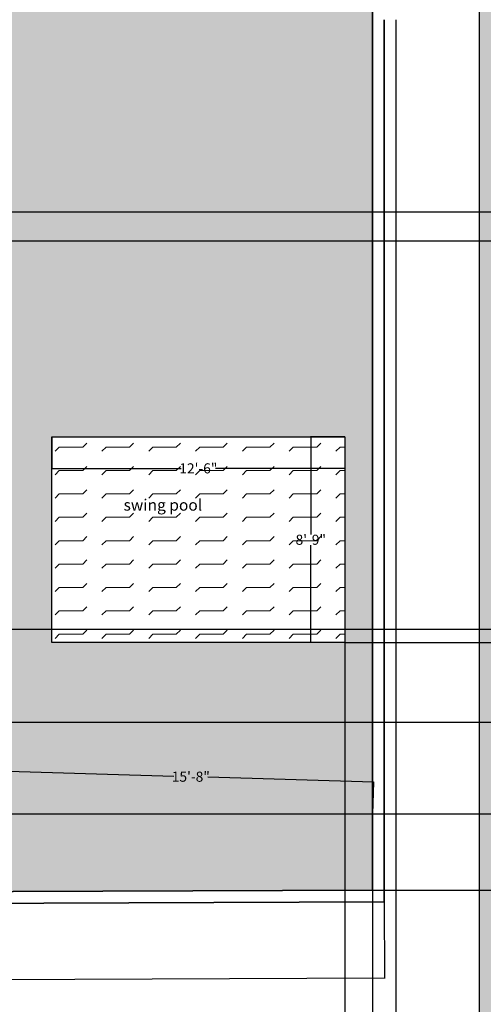
# Model space of a CAD drawing. Units: inches. Extents: x -157 to 1464, y -361 to 1077.
# Tile 7 of 9: x 676 to 913, y 14 to 519. Entities that reach past the tile are written whole.
import ezdxf

# ---------------------------------------------------------------- set-up
doc = ezdxf.new("R2010")
doc.units = ezdxf.units.IN
doc.header["$MEASUREMENT"] = 0
for name, color, linetype, lineweight in [('A-ANNO-DIMS', 2, 'Continuous', 18), ('C-ANNO-DIMS', 2, 'Continuous', 18), ('C-ANNO-TEXT', 7, 'Continuous', 18), ('C-POOL-PATT', 143, 'Continuous', 13), ('C-PROP', 7, 'Continuous', 35), ('C-ROAD', 7, 'Continuous', 25), ('C-ROAD-PATT', 8, 'Continuous', 13), ('C-SITE-POOL', 4, 'Continuous', 25), ('L-GRND-PATT', 8, 'Continuous', 13)]:
    doc.layers.add(name, color=color, linetype=linetype, lineweight=lineweight)
doc.styles.get("Standard").update_dxf_attribs({"font": 'arial.ttf'})
doc.dimstyles.new('Annotative', dxfattribs={"dimscale": 0, "dimtxt": 5.18, "dimasz": 0.18, "dimexe": 0.18, "dimexo": 0.0625, "dimgap": 0.09, "dimtad": 0, "dimtih": 1, "dimtoh": 1, "dimdec": 0, "dimzin": 0, "dimdsep": 46, "dimlunit": 3, "dimtxsty": 'Standard', "dimcen": 0.09, "dimadec": 0, "dimazin": 0, "dimtfac": 1, "dimtdec": 0, "dimtofl": 0, "dimtmove": 0, "dimatfit": 3, "dimfxl": 1, "dimtolj": 1, "dimtzin": 0, "dimarcsym": 0})

# ---------------------------------------------------------------- blocks, each defined once
blk = doc.blocks.new('*D14')
at = {"layer": 'C-ANNO-DIMS', "color": 0, "lineweight": -2, "transparency": 16777216}
for p, q in [((862.57, 66.62), (862.72, 27.26)), ((251.33, 64.28), (251.48, 24.92)), ((251.66, 25.1), (546.1, 26.23)), ((862.54, 27.44), (568.1, 26.31))]:
    blk.add_line(p, q, dxfattribs=at)
at = {"layer": 'C-ANNO-DIMS', "color": 0, "transparency": 16777216}
for points in [[(862.54, 27.47), (862.54, 27.41), (862.72, 27.44)], [(251.66, 25.13), (251.66, 25.07), (251.48, 25.1)]]:
    blk.add_solid(points, dxfattribs=at)
at = {"layer": 'Defpoints', "color": 0, "transparency": 16777216}
for p in [(862.57, 66.68), (251.33, 64.34), (862.72, 27.44)]:
    blk.add_point(p, dxfattribs=at)
at = {"layer": 'C-ANNO-DIMS', "color": 0, "transparency": 16777216, "insert": (557.1, 26.27), "char_height": 5.18, "attachment_point": 5}
blk.add_mtext('\\A1;50\'-11"', dxfattribs=at)
blk = doc.blocks.new('*D15')
at = {"layer": 'C-ANNO-DIMS', "color": 0, "lineweight": -2, "transparency": 16777216}
for p, q in [((692.18, 305.18), (692.18, 288.97)), ((842.44, 305.18), (842.44, 288.97)), ((692.36, 289.15), (758.57, 289.15)), ((842.26, 289.15), (776.05, 289.15))]:
    blk.add_line(p, q, dxfattribs=at)
at = {"layer": 'C-ANNO-DIMS', "color": 0, "transparency": 16777216}
for points in [[(692.36, 289.18), (692.36, 289.12), (692.18, 289.15)], [(842.26, 289.18), (842.26, 289.12), (842.44, 289.15)]]:
    blk.add_solid(points, dxfattribs=at)
at = {"layer": 'Defpoints', "color": 0, "transparency": 16777216}
for p in [(692.18, 305.24), (842.44, 305.24), (842.44, 289.15)]:
    blk.add_point(p, dxfattribs=at)
at = {"layer": 'C-ANNO-DIMS', "color": 0, "transparency": 16777216, "insert": (767.31, 289.15), "char_height": 5.18, "attachment_point": 5}
blk.add_mtext('\\A1;12\'-6"', dxfattribs=at)
blk = doc.blocks.new('*D16')
at = {"layer": 'C-ANNO-DIMS', "color": 0, "lineweight": -2, "transparency": 16777216}
for p, q in [((842.38, 305.24), (824.79, 305.24)), ((824.97, 305.06), (824.97, 255.24)), ((824.97, 199.96), (824.97, 249.77)), ((842.38, 199.78), (824.79, 199.78))]:
    blk.add_line(p, q, dxfattribs=at)
at = {"layer": 'C-ANNO-DIMS', "color": 0, "transparency": 16777216}
for points in [[(824.94, 305.06), (825, 305.06), (824.97, 305.24)], [(824.94, 199.96), (825, 199.96), (824.97, 199.78)]]:
    blk.add_solid(points, dxfattribs=at)
at = {"layer": 'Defpoints', "color": 0, "transparency": 16777216}
for p in [(842.44, 305.24), (824.97, 199.78), (842.44, 199.78)]:
    blk.add_point(p, dxfattribs=at)
at = {"layer": 'C-ANNO-DIMS', "color": 0, "transparency": 16777216, "insert": (824.97, 252.51), "char_height": 5.18, "attachment_point": 5}
blk.add_mtext('\\A1;8\'-9"', dxfattribs=at)
blk = doc.blocks.new('*D56')
at = {"layer": 'C-ANNO-DIMS', "color": 0, "lineweight": -2, "transparency": 16777216}
for p, q in [((668.97, 111.92), (669.64, 133.96)), ((669.82, 133.77), (754.7, 131.17)), ((857.06, 128.03), (772.18, 130.63)), ((856.57, 106.17), (857.25, 128.21))]:
    blk.add_line(p, q, dxfattribs=at)
at = {"layer": 'C-ANNO-DIMS', "color": 0, "transparency": 16777216}
for points in [[(669.82, 133.8), (669.82, 133.74), (669.64, 133.78)], [(857.06, 128.06), (857.06, 128), (857.24, 128.03)]]:
    blk.add_solid(points, dxfattribs=at)
at = {"layer": 'Defpoints', "color": 0, "transparency": 16777216}
for p in [(857.24, 128.03), (668.97, 111.86), (856.57, 106.11)]:
    blk.add_point(p, dxfattribs=at)
at = {"layer": 'C-ANNO-DIMS', "color": 0, "transparency": 16777216, "insert": (763.44, 130.9), "char_height": 5.18, "attachment_point": 5}
blk.add_mtext('\\A1;15\'-8"', dxfattribs=at)
blk = doc.blocks.new('*D64')
at = {"layer": 'A-ANNO-DIMS', "color": 0, "lineweight": -2, "transparency": 16777216}
for p, q in [((842.44, 199.71), (842.44, -357.73)), ((856.57, 72.59), (856.57, -357.73)), ((842.62, -357.55), (842.77, -357.55)), ((856.39, -357.55), (856.24, -357.55))]:
    blk.add_line(p, q, dxfattribs=at)
at = {"layer": 'A-ANNO-DIMS', "color": 0, "transparency": 16777216}
for points in [[(842.62, -357.52), (842.62, -357.58), (842.44, -357.55)], [(856.39, -357.52), (856.39, -357.58), (856.57, -357.55)]]:
    blk.add_solid(points, dxfattribs=at)
at = {"layer": 'Defpoints', "color": 0, "transparency": 16777216}
for p in [(842.44, 199.78), (856.57, 72.66), (856.57, -357.55)]:
    blk.add_point(p, dxfattribs=at)
at = {"layer": 'A-ANNO-DIMS', "color": 0, "transparency": 16777216, "insert": (849.51, -357.55), "char_height": 5.18, "attachment_point": 5}
blk.add_mtext('\\A1;1\'-2"', dxfattribs=at)
blk = doc.blocks.new('*D65')
at = {"layer": 'A-ANNO-DIMS', "color": 0, "lineweight": -2, "transparency": 16777216}
for p, q in [((842.5, 199.78), (1397.57, 199.78)), ((1397.39, 199.6), (1397.39, 138.95)), ((1397.39, 72.84), (1397.39, 133.48)), ((856.63, 72.66), (1397.57, 72.66))]:
    blk.add_line(p, q, dxfattribs=at)
at = {"layer": 'A-ANNO-DIMS', "color": 0, "transparency": 16777216}
for points in [[(1397.36, 199.6), (1397.42, 199.6), (1397.39, 199.78)], [(1397.36, 72.84), (1397.42, 72.84), (1397.39, 72.66)]]:
    blk.add_solid(points, dxfattribs=at)
at = {"layer": 'Defpoints', "color": 0, "transparency": 16777216}
for p in [(842.44, 199.78), (856.57, 72.66), (1397.39, 72.66)]:
    blk.add_point(p, dxfattribs=at)
at = {"layer": 'A-ANNO-DIMS', "color": 0, "transparency": 16777216, "insert": (1397.39, 136.22), "char_height": 5.18, "attachment_point": 5}
blk.add_mtext('\\A1;10\'-7"', dxfattribs=at)
blk = doc.blocks.new('*D69')
at = {"layer": 'A-ANNO-DIMS', "color": 0, "lineweight": -2, "transparency": 16777216}
for p, q in [((856.57, 519.36), (856.57, -357.73)), ((868.57, 519.36), (868.57, -357.73)), ((856.75, -357.55), (868.39, -357.55)), ((868.57, -357.55), (868.75, -357.55))]:
    blk.add_line(p, q, dxfattribs=at)
at = {"layer": 'A-ANNO-DIMS', "color": 0, "transparency": 16777216}
for points in [[(856.75, -357.52), (856.75, -357.58), (856.57, -357.55)], [(868.39, -357.52), (868.39, -357.58), (868.57, -357.55)]]:
    blk.add_solid(points, dxfattribs=at)
at = {"layer": 'Defpoints', "color": 0, "transparency": 16777216}
for p in [(856.57, 519.42), (868.57, 519.42), (868.57, -357.55)]:
    blk.add_point(p, dxfattribs=at)
at = {"layer": 'A-ANNO-DIMS', "color": 0, "transparency": 16777216, "insert": (875.48, -357.55), "char_height": 5.18, "attachment_point": 5}
blk.add_mtext('\\A1;1\'-0"', dxfattribs=at)
blk = doc.blocks.new('*D74')
at = {"layer": 'A-ANNO-DIMS', "color": 0, "lineweight": -2, "transparency": 16777216}
for p, q in [((597.03, 158.9), (1397.57, 158.9)), ((1397.39, 158.72), (1397.39, 138.11)), ((1397.39, 112.04), (1397.39, 132.64)), ((597.03, 111.86), (1397.57, 111.86))]:
    blk.add_line(p, q, dxfattribs=at)
at = {"layer": 'A-ANNO-DIMS', "color": 0, "transparency": 16777216}
for points in [[(1397.36, 158.72), (1397.42, 158.72), (1397.39, 158.9)], [(1397.36, 112.04), (1397.42, 112.04), (1397.39, 111.86)]]:
    blk.add_solid(points, dxfattribs=at)
at = {"layer": 'Defpoints', "color": 0, "transparency": 16777216}
for p in [(596.97, 158.9), (1397.39, 158.9), (596.97, 111.86)]:
    blk.add_point(p, dxfattribs=at)
at = {"layer": 'A-ANNO-DIMS', "color": 0, "transparency": 16777216, "insert": (1397.39, 135.38), "char_height": 5.18, "attachment_point": 5}
blk.add_mtext('\\A1;3\'-11"', dxfattribs=at)
blk = doc.blocks.new('*D76')
at = {"layer": 'A-ANNO-DIMS', "color": 0, "lineweight": -2, "transparency": 16777216}
for p, q in [((597.03, 420.86), (1397.57, 420.86)), ((1397.39, 420.68), (1397.39, 416.1)), ((1397.39, 406.04), (1397.39, 410.62)), ((597.03, 405.86), (1397.57, 405.86))]:
    blk.add_line(p, q, dxfattribs=at)
at = {"layer": 'A-ANNO-DIMS', "color": 0, "transparency": 16777216}
for points in [[(1397.36, 420.68), (1397.42, 420.68), (1397.39, 420.86)], [(1397.36, 406.04), (1397.42, 406.04), (1397.39, 405.86)]]:
    blk.add_solid(points, dxfattribs=at)
at = {"layer": 'Defpoints', "color": 0, "transparency": 16777216}
for p in [(596.97, 420.86), (1397.39, 420.86), (596.97, 405.86)]:
    blk.add_point(p, dxfattribs=at)
at = {"layer": 'A-ANNO-DIMS', "color": 0, "transparency": 16777216, "insert": (1397.39, 413.36), "char_height": 5.18, "attachment_point": 5}
blk.add_mtext('\\A1;1\'-3"', dxfattribs=at)
blk = doc.blocks.new('*D83')
at = {"layer": 'A-ANNO-DIMS', "color": 0, "lineweight": -2, "transparency": 16777216}
for p, q in [((652.31, 206.63), (1397.57, 206.63)), ((1397.39, 206.45), (1397.39, 161.94)), ((1397.39, 112.04), (1397.39, 156.56)), ((597.03, 111.86), (1397.57, 111.86))]:
    blk.add_line(p, q, dxfattribs=at)
at = {"layer": 'A-ANNO-DIMS', "color": 0, "transparency": 16777216}
for points in [[(1397.36, 206.45), (1397.42, 206.45), (1397.39, 206.63)], [(1397.36, 112.04), (1397.42, 112.04), (1397.39, 111.86)]]:
    blk.add_solid(points, dxfattribs=at)
at = {"layer": 'Defpoints', "color": 0, "transparency": 16777216}
for p in [(652.25, 206.63), (1397.39, 206.63), (596.97, 111.86)]:
    blk.add_point(p, dxfattribs=at)
at = {"layer": 'A-ANNO-DIMS', "color": 0, "transparency": 16777216, "insert": (1397.39, 159.25), "char_height": 5.18, "attachment_point": 5}
blk.add_mtext('\\A1;7\'-11"', dxfattribs=at)

msp = doc.modelspace()

# ---------------------------------------------------------------- hatches: boundary and pattern name
at = {"layer": 'C-POOL-PATT'}
h = msp.add_hatch(dxfattribs=at)
h.set_pattern_fill('FLEX', color=256, scale=48)
h.paths.add_polyline_path([(842.44, 305.24), (692.18, 305.24), (692.18, 199.78), (842.44, 199.78)])
at = {"layer": 'C-ROAD-PATT'}
h = msp.add_hatch(color=256, dxfattribs=at)
h.dxf.hatch_style = 1
h.paths.add_polyline_path([(1091.28, 858.84), (31.23, 858.84), (31.23, 838.38), (161.57, 774.56), (996.76, 774.56), (996.76, -105.32), (1027.51, -42.52), (1027.51, -185.11), (1027.51, -287.61), (1091.28, -186.19)])
h.paths.add_polyline_path([(899.55, 208.71), (1098.57, 208.71), (1098.57, 279.4), (899.55, 279.4)], flags=9)
h = msp.add_hatch(color=256, dxfattribs=at)
h.dxf.hatch_style = 1
h.paths.add_polyline_path([(990.76, 768.56), (31.23, 768.56), (-71.27, 768.56), (31.23, 704.11), (31.23, 678.84), (911.28, 678.84), (911.28, -185.11), (957.69, -185.11), (990.76, -117.57)])
h.paths.add_polyline_path([(899.55, 208.71), (1098.57, 208.71), (1098.57, 279.4), (899.55, 279.4)], flags=9)
h.paths.add_polyline_path([(645.57, 707.88), (844.59, 707.88), (844.59, 778.57), (645.57, 778.57)], flags=9)
h.paths.add_polyline_path([(892.1, 580.27), (940.38, 580.27), (940.38, 592.3), (892.1, 592.3)], flags=25)
at = {"layer": 'L-GRND-PATT'}
h = msp.add_hatch(dxfattribs=at)
h.set_pattern_fill('GRAVEL', color=256, scale=26)
h.set_pattern_definition([(228.01279, (18.72, 26), (-208, -234), [3.49794, -346.2963]), (184.96974, (16.38, 23.4), (312, 26), [6.00257, -594.25404]), (132.51045, (10.4, 22.88), (260, -286), [4.2325, -419.01685]), (267.27369, (0.26, 16.38), (26, 520), [5.4662, -541.1525]), (292.83365, (0, 10.92), (-130, 312), [5.36003, -530.6437]), (357.27369, (2.08, 5.98), (-520, 26), [5.4662, -541.1525]), (37.69424, (7.54, 5.72), (-338, -260), [7.22875, -715.64606]), (72.25533, (13.26, 10.14), (182, 572), [6.8247, -675.64436]), (121.42957, (15.34, 16.64), (-208, 338), [5.4847, -542.9859]), (175.23636, (12.48, 21.32), (286, -26), [6.26163, -306.81983]), (222.39744, (6.24, 21.84), (-312, -286), [8.09765, -801.66775]), (138.81407, (26, 16.12), (-182, 156), [2.76383, -273.61997]), (171.46923, (23.92, 17.94), (338, -52), [5.25816, -520.5593]), (225, (18.72, 18.72), (-3e-15, -26), [3.67695, -33.0926]), (203.1986, (16.9, 21.84), (130, 52), [1.9801, -196.03]), (291.8014, (15.08, 21.06), (-26, 78), [2.8003, -137.214]), (30.96376, (16.12, 18.46), (78, 52), [4.54815, -147.0566]), (161.56505, (20.02, 20.8), (52, -26), [3.28877, -78.93045]), (16.38954, (0, 21.06), (260, 78), [4.6072, -456.11397]), (70.34618, (4.42, 22.36), (-104, -286), [3.8652, -382.6526]), (293.1986, (20.02, 26), (-52, 130), [3.9602, -194.0499]), (343.61046, (21.58, 22.36), (-260, 78), [4.6072, -456.11397]), (339.44395, (0, 4.94), (-130, 52), [4.4429, -217.7012]), (294.77514, (4.16, 3.38), (-130, 286), [3.72263, -368.5407]), (66.8014, (20.28, 0), (52, 130), [3.9602, -194.0499]), (17.35402, (21.84, 3.64), (-338, -104), [4.3584, -431.481]), (69.44395, (7.54, 0), (-52, -130), [2.22144, -219.92266]), (101.30993, (18.72, 0), (-26, 104), [1.32574, -131.24877]), (165.96376, (18.46, 1.3), (78, -26), [5.36003, -101.8407]), (186.009, (13.26, 2.6), (260, 26), [4.9673, -491.762]), (303.6901, (16.12, 16.12), (-26, 52), [3.7498, -89.99456]), (353.15723, (18.2, 13), (442, -52), [6.54664, -648.11663]), (60.9454, (24.7, 12.22), (-104, -182), [2.67686, -265.00953]), (90, (26, 14.56), (-26, 26), [1.56, -24.44]), (120.25644, (12.74, 3.38), (104, -182), [3.61202, -357.5915]), (48.01279, (10.92, 6.5), (208, 234), [6.99587, -342.79835]), (0, (15.6, 11.7), (26, 26), [6.76, -19.24]), (325.30485, (22.36, 11.7), (260, -182), [4.11096, -406.98513]), (254.0546, (25.74, 9.36), (-26, -104), [3.78565, -185.4972]), (207.64598, (24.7, 5.72), (-494, -260), [6.1637, -610.20633]), (175.42608, (19.24, 2.86), (-338, 26), [6.52077, -645.5559])])
h.paths.add_polyline_path([(856.57, 645.71), (257.33, 643.42), (257.33, 70.37), (856.57, 72.66)])
h.paths.add_polyline_path([(668.97, 111.86), (596.97, 111.86), (298.97, 111.86), (298.97, 420.86), (298.97, 492.86), (427.97, 492.86), (668.97, 492.86)], flags=16)
h.paths.add_polyline_path([(842.44, 305.24), (842.44, 199.78), (692.18, 199.78), (692.18, 305.24)], flags=16)
h.paths.add_polyline_path([(596.97, 369.86), (596.97, 158.9), (587.97, 158.9), (587.97, 120.86), (485.97, 120.86), (485.97, 203.86), (468.97, 203.86), (468.97, 198.86), (480.97, 198.86), (480.97, 120.86), (465.97, 120.86), (465.97, 111.86), (447.97, 111.86), (447.97, 120.86), (432.97, 120.86), (432.97, 198.86), (438.97, 198.86), (438.97, 203.86), (432.97, 203.86), (432.97, 226.86), (427.97, 226.86), (427.97, 120.86), (307.97, 120.86), (307.97, 146.36), (298.97, 146.36), (298.97, 194.36), (307.97, 194.36), (307.97, 267.86), (427.97, 267.86), (427.97, 262.86), (432.97, 262.86), (432.97, 277.86), (427.97, 277.86), (427.97, 272.86), (307.97, 272.86), (307.97, 276.53), (298.97, 276.53), (298.97, 324.53), (307.97, 324.53), (307.97, 411.86), (427.97, 411.86), (427.97, 313.86), (432.97, 313.86), (432.97, 411.86), (463.95, 411.86), (463.95, 420.86), (334.97, 420.86), (334.97, 456.86), (427.97, 456.86), (427.97, 420.86), (546.97, 420.86), (582.97, 420.86), (596.97, 420.86), (596.97, 405.86)], flags=0)
h.paths.add_polyline_path([(596.97, 369.86), (587.97, 369.86), (587.97, 324), (596.97, 324), (596.97, 276), (587.97, 276), (587.97, 369.86), (587.97, 405.86), (587.97, 411.86), (582.97, 411.86), (546.97, 411.86), (546.97, 420.86), (564.97, 416.36), (582.97, 420.86), (582.97, 411.86), (587.97, 411.86), (587.97, 405.86), (596.97, 405.86), (592.47, 387.86)], flags=0)
h.paths.add_polyline_path([(468.97, 203.86), (468.97, 198.86), (438.97, 198.86), (438.97, 203.86)], flags=0)
h.paths.add_polyline_path([(267.35, 260.99), (288.37, 260.99), (288.37, 271.66), (267.35, 271.66)], flags=24)
h.paths.add_polyline_path([(435.51, 88.48), (460.55, 88.48), (460.55, 99.15), (435.51, 99.15)], flags=24)
h.paths.add_polyline_path([(315.69, 188.99), (336.72, 188.99), (336.72, 199.66), (315.69, 199.66)], flags=8)
h.paths.add_polyline_path([(361.73, 141.9), (373.75, 141.9), (373.75, 152.57), (361.73, 152.57)], flags=8)
h.paths.add_polyline_path([(430.38, 154.49), (447.38, 154.49), (447.38, 165.16), (430.38, 165.16)], flags=8)
h.paths.add_polyline_path([(451.09, 165.32), (468.09, 165.32), (468.09, 175.99), (451.09, 175.99)], flags=8)
h.paths.add_polyline_path([(361.73, 305.06), (373.75, 305.06), (373.75, 315.74), (361.73, 315.74)], flags=8)
h.paths.add_polyline_path([(316.13, 336.94), (337.15, 336.94), (337.15, 347.62), (316.13, 347.62)], flags=8)
h.paths.add_polyline_path([(484.07, 423.56), (492.07, 423.56), (492.07, 434.24), (484.07, 434.24)], flags=8)
h.paths.add_polyline_path([(560.99, 428.52), (568.98, 428.52), (568.98, 439.19), (560.99, 439.19)], flags=8)
h.paths.add_polyline_path([(528.49, 131.95), (545.49, 131.95), (545.49, 142.62), (528.49, 142.62)], flags=8)
h.paths.add_polyline_path([(564.53, 188.99), (585.55, 188.99), (585.55, 199.66), (564.53, 199.66)], flags=8)

# ---------------------------------------------------------------- linework, layer by layer
at = {"layer": 'C-PROP'}
msp.add_lwpolyline([(862.57, 615.42), (862.57, 651.74), (251.33, 649.4), (251.33, 64.34), (862.57, 66.68), (862.57, 519.42)], dxfattribs=at)
msp.add_lwpolyline([(257.33, 70.37), (856.57, 72.66), (856.57, 645.71), (257.33, 643.42)], close=True, dxfattribs=at)
at = {"layer": 'C-ROAD'}
msp.add_line((911.28, 678.84), (911.28, -185.11), dxfattribs=at)
at = {"layer": 'C-SITE-POOL'}
msp.add_lwpolyline([(692.18, 305.24), (842.44, 305.24), (842.44, 199.78), (692.18, 199.78)], close=True, dxfattribs=at)

# ---------------------------------------------------------------- texts
at = {"layer": 'C-ANNO-TEXT', "insert": (728.96, 273.27), "char_height": 5.84, "attachment_point": 1}
msp.add_mtext_dynamic_manual_height_columns('swing pool', width=87.358, gutter_width=29.2, heights=[13.12], dxfattribs=at)

# ---------------------------------------------------------------- dimensions: what is measured, and where the dimension line sits
at = {"layer": 'A-ANNO-DIMS'}
for base, p1, p2, picture, middle in [((868.57, -357.55), (856.57, 519.42), (868.57, 519.42), '*D69', (875.48, -357.55)), ((856.57, -357.55), (842.44, 199.78), (856.57, 72.66), '*D64', (849.51, -357.55))]:
    dim = msp.add_linear_dim(base=base, p1=p1, p2=p2, dimstyle='Annotative', override={"dimscale": 1, "dimdec": 1, "dimzin": 1, "dimlunit": 4, "dimfrac": 2}, dxfattribs=at)
    dim.commit()
    dim.dimension.update_dxf_attribs({"geometry": picture, "text_midpoint": middle})
for base, p1, p2, picture, middle in [((1397.39, 420.86), (596.97, 405.86), (596.97, 420.86), '*D76', (1397.39, 413.36)), ((1397.39, 206.63), (596.97, 111.86), (652.25, 206.63), '*D83', (1397.39, 159.25)), ((1397.39, 72.66), (842.44, 199.78), (856.57, 72.66), '*D65', (1397.39, 136.22)), ((1397.39, 158.9), (596.97, 111.86), (596.97, 158.9), '*D74', (1397.39, 135.38))]:
    dim = msp.add_linear_dim(base=base, p1=p1, p2=p2, angle=90, dimstyle='Annotative', override={"dimscale": 1, "dimdec": 1, "dimzin": 1, "dimlunit": 4, "dimfrac": 2}, dxfattribs=at)
    dim.commit()
    dim.dimension.update_dxf_attribs({"geometry": picture, "text_midpoint": middle})
at = {"layer": 'C-ANNO-DIMS'}
dim = msp.add_linear_dim(base=(842.44, 289.15), p1=(692.18, 305.24), p2=(842.44, 305.24), dimstyle='Annotative', override={"dimclrd": 0, "dimclre": 0, "dimclrt": 0}, dxfattribs=at)
dim.commit()
dim.dimension.update_dxf_attribs({"geometry": '*D15', "text_midpoint": (767.31, 289.15)})
dim = msp.add_linear_dim(base=(824.97, 199.78), p1=(842.44, 305.24), p2=(842.44, 199.78), angle=90, dimstyle='Annotative', override={"dimclrd": 0, "dimclre": 0, "dimclrt": 0}, dxfattribs=at)
dim.commit()
dim.dimension.update_dxf_attribs({"geometry": '*D16', "text_midpoint": (824.97, 252.51)})
for p1, p2, distance, picture, middle in [((668.97, 111.86), (856.57, 106.11), 21.93, '*D56', (763.44, 130.9)), ((251.33, 64.34), (862.57, 66.68), -39.24, '*D14', (557.1, 26.27))]:
    dim = msp.add_aligned_dim(p1=p1, p2=p2, distance=distance, dimstyle='Annotative', override={"dimclrd": 0, "dimclre": 0, "dimclrt": 0}, dxfattribs=at)
    dim.commit()
    dim.dimension.update_dxf_attribs({"geometry": picture, "text_midpoint": middle})

doc.saveas('drawing.dxf')
